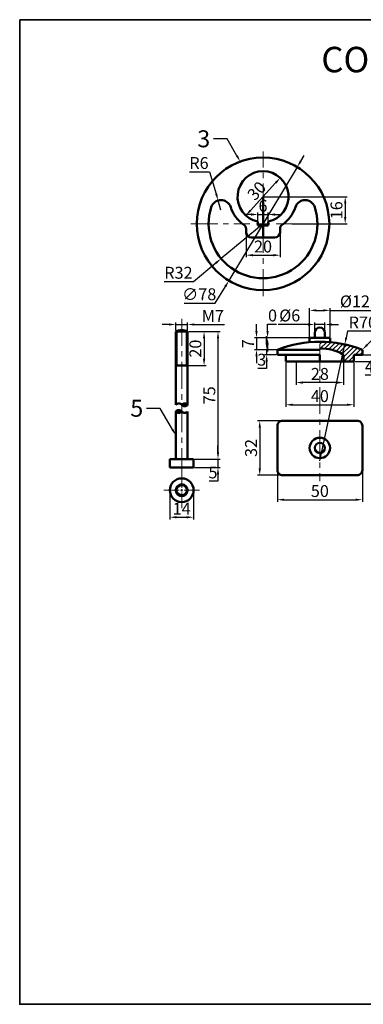
# Model space of a CAD drawing. Units: millimetres. Extents: x 214 to 813, y -258 to 321.
# Tile 1 of 4: x 214 to 416, y -258 to 321. Entities that reach past the tile are written whole.
import ezdxf
from ezdxf import colors
from ezdxf.entities.mleader import LeaderData, LeaderLine
from ezdxf.math import Vec2, Vec3

# ---------------------------------------------------------------- set-up
doc = ezdxf.new("R2010")
doc.units = ezdxf.units.MM
doc.header["$LTSCALE"] = 0.5
doc.linetypes.add('CENTER', pattern=[50.8, 31.75, -6.35, 6.35, -6.35])
for name, color, linetype, lineweight in [('M-CNTR', 1, 'CENTER', 18), ('M-DIMS', 2, 'Continuous', 25), ('M-HATC', 8, 'Continuous', 18), ('M-OUTL', 7, 'Continuous', 50), ('M-TTLB', 7, 'Continuous', 35)]:
    doc.layers.add(name, color=color, linetype=linetype, lineweight=lineweight)
doc.styles.get("Standard").update_dxf_attribs({"font": 'arial.ttf'})
doc.dimstyles.new('ISO-25', dxfattribs={"dimtxt": 7, "dimasz": 4, "dimexe": 1.25, "dimexo": 0.625, "dimtad": 1, "dimtoh": 1, "dimtxsty": 'Standard', "dimcen": 2.5, "dimadec": 0, "dimazin": 0, "dimtfac": 1, "dimtmove": 0, "dimatfit": 3, "dimfxl": 1, "dimarcsym": 0})
pattern_1 = [(45, (-3.20253, -20.17053), (-0.2245064, 0.2245064), [])]

# ---------------------------------------------------------------- blocks, each defined once
blk = doc.blocks.new('*U1')
at = {"layer": 'M-CNTR', "color": 0, "transparency": 16777216}
for p, q in [((0, 7.8), (0, 42.5)), ((-42.5, 0), (-7.8, 0)), ((7.8, 0), (42.5, 0)), ((0, -42.5), (0, -7.8))]:
    blk.add_line(p, q, dxfattribs=at)
at = {"layer": 'M-CNTR', "color": 0, "linetype": 'Continuous', "transparency": 16777216}
for p, q in [((-3.9, 0), (3.9, 0)), ((0, -3.9), (0, 3.9))]:
    blk.add_line(p, q, dxfattribs=at)
blk = doc.blocks.new('*D26')
at = {"layer": 'Defpoints', "color": 0, "ltscale": 0.5, "transparency": 16777216}
for p in [(367.44, 228.4), (347.21, 206.25), (347.21, 206.25)]:
    blk.add_point(p, dxfattribs=at)
at = {"layer": 'M-DIMS', "color": 0, "lineweight": -2, "ltscale": 0.5, "transparency": 16777216}
for p, q in [((366.98, 228.82), (366.52, 229.24)), ((364.75, 225.45), (349.91, 209.2)), ((346.75, 206.67), (346.29, 207.09))]:
    blk.add_line(p, q, dxfattribs=at)
at = {"layer": 'M-DIMS', "color": 0, "ltscale": 0.5, "transparency": 16777216}
for points in [[(364.25, 225.89), (365.24, 225), (367.44, 228.4)], [(349.42, 209.65), (350.4, 208.75), (347.21, 206.25)]]:
    blk.add_solid(points, dxfattribs=at)
at = {"layer": 'M-DIMS', "color": 0, "ltscale": 0.5, "transparency": 16777216, "insert": (354.23, 220.16), "char_height": 7, "attachment_point": 5, "rotation": 47.59957}
blk.add_mtext('30', dxfattribs=at)
blk = doc.blocks.new('*D27')
at = {"layer": 'Defpoints', "color": 0, "ltscale": 0.5, "transparency": 16777216}
for p in [(360.33, 206.82), (354.33, 202.63), (360.33, 202.63)]:
    blk.add_point(p, dxfattribs=at)
at = {"layer": 'M-DIMS', "color": 0, "lineweight": -2, "ltscale": 0.5, "transparency": 16777216}
for p, q in [((350.33, 206.82), (346.33, 206.82)), ((354.33, 203.25), (354.33, 208.07)), ((354.33, 206.82), (360.33, 206.82)), ((360.33, 203.25), (360.33, 208.07)), ((364.33, 206.82), (368.33, 206.82))]:
    blk.add_line(p, q, dxfattribs=at)
at = {"layer": 'M-DIMS', "color": 0, "ltscale": 0.5, "transparency": 16777216}
for points in [[(350.33, 207.49), (350.33, 206.16), (354.33, 206.82)], [(364.33, 207.49), (364.33, 206.16), (360.33, 206.82)]]:
    blk.add_solid(points, dxfattribs=at)
at = {"layer": 'M-DIMS', "color": 0, "ltscale": 0.5, "transparency": 16777216, "insert": (357.33, 211.02), "char_height": 7, "attachment_point": 5}
blk.add_mtext('6', dxfattribs=at)
blk = doc.blocks.new('*D28')
at = {"layer": 'Defpoints', "color": 0, "ltscale": 0.5, "transparency": 16777216}
for p in [(357.33, 201.32), (332.71, 180.88)]:
    blk.add_point(p, dxfattribs=at)
at = {"layer": 'M-DIMS', "color": 0, "lineweight": -2, "ltscale": 0.5, "transparency": 16777216}
for p, q in [((357.33, 201.32), (332.71, 180.88)), ((316.5, 167.42), (329.63, 178.32)), ((299.22, 167.42), (316.5, 167.42))]:
    blk.add_line(p, q, dxfattribs=at)
at = {"layer": 'M-DIMS', "color": 0, "ltscale": 0.5, "transparency": 16777216}
blk.add_solid([(329.21, 178.84), (330.06, 177.81), (332.71, 180.88)], dxfattribs=at)
at = {"layer": 'M-DIMS', "color": 0, "ltscale": 0.5, "transparency": 16777216, "insert": (307.55, 171.62), "char_height": 7, "attachment_point": 5}
blk.add_mtext('R32', dxfattribs=at)
blk = doc.blocks.new('*D29')
at = {"layer": 'Defpoints', "color": 0, "ltscale": 0.5, "transparency": 16777216}
for p in [(377.42, 234.75), (337.24, 167.89)]:
    blk.add_point(p, dxfattribs=at)
at = {"layer": 'M-DIMS', "color": 0, "lineweight": -2, "ltscale": 0.5, "transparency": 16777216}
for p, q in [((379.48, 238.18), (381.54, 241.61)), ((377.42, 234.75), (337.24, 167.89)), ((329.24, 154.57), (335.18, 164.46)), ((310.95, 154.57), (329.24, 154.57))]:
    blk.add_line(p, q, dxfattribs=at)
at = {"layer": 'M-DIMS', "color": 0, "ltscale": 0.5, "transparency": 16777216}
for points in [[(378.91, 238.52), (380.05, 237.84), (377.42, 234.75)], [(334.61, 164.81), (335.75, 164.12), (337.24, 167.89)]]:
    blk.add_solid(points, dxfattribs=at)
at = {"layer": 'M-DIMS', "color": 0, "ltscale": 0.5, "transparency": 16777216, "insert": (319.78, 158.97), "char_height": 7, "attachment_point": 5}
blk.add_mtext('∅78', dxfattribs=at)
blk = doc.blocks.new('*D30')
at = {"layer": 'Defpoints', "color": 0, "ltscale": 0.5, "transparency": 16777216}
for p in [(347.33, 196.32), (367.33, 196.32), (367.33, 182.87)]:
    blk.add_point(p, dxfattribs=at)
at = {"layer": 'M-DIMS', "color": 0, "lineweight": -2, "ltscale": 0.5, "transparency": 16777216}
for p, q in [((347.33, 195.7), (347.33, 181.62)), ((367.33, 195.7), (367.33, 181.62)), ((351.33, 182.87), (363.33, 182.87))]:
    blk.add_line(p, q, dxfattribs=at)
at = {"layer": 'M-DIMS', "color": 0, "ltscale": 0.5, "transparency": 16777216}
for points in [[(351.33, 183.54), (351.33, 182.21), (347.33, 182.87)], [(363.33, 183.54), (363.33, 182.21), (367.33, 182.87)]]:
    blk.add_solid(points, dxfattribs=at)
at = {"layer": 'M-DIMS', "color": 0, "ltscale": 0.5, "transparency": 16777216, "insert": (357.33, 187.07), "char_height": 7, "attachment_point": 5}
blk.add_mtext('20', dxfattribs=at)
blk = doc.blocks.new('*D31')
at = {"layer": 'Defpoints', "color": 0, "ltscale": 0.5, "transparency": 16777216}
for p in [(330.9, 215.08), (332.59, 209.32)]:
    blk.add_point(p, dxfattribs=at)
at = {"layer": 'M-DIMS', "color": 0, "lineweight": -2, "ltscale": 0.5, "transparency": 16777216}
for p, q in [((314, 232.03), (325.91, 232.03)), ((325.91, 232.03), (329.77, 218.92)), ((332.59, 209.32), (330.9, 215.08))]:
    blk.add_line(p, q, dxfattribs=at)
at = {"layer": 'M-DIMS', "color": 0, "ltscale": 0.5, "transparency": 16777216}
blk.add_solid([(330.41, 219.1), (329.13, 218.73), (330.9, 215.08)], dxfattribs=at)
at = {"layer": 'M-DIMS', "color": 0, "ltscale": 0.5, "transparency": 16777216, "insert": (319.64, 236.23), "char_height": 7, "attachment_point": 5}
blk.add_mtext('R6', dxfattribs=at)
blk = doc.blocks.new('*D32')
at = {"layer": 'Defpoints', "color": 0, "ltscale": 0.5, "transparency": 16777216}
for p in [(357.33, 217.32), (373.64, 201.32), (405.66, 201.32)]:
    blk.add_point(p, dxfattribs=at)
at = {"layer": 'M-DIMS', "color": 0, "lineweight": -2, "ltscale": 0.5, "transparency": 16777216}
for p, q in [((357.95, 217.32), (406.91, 217.32)), ((405.66, 213.32), (405.66, 205.32)), ((374.27, 201.32), (406.91, 201.32))]:
    blk.add_line(p, q, dxfattribs=at)
at = {"layer": 'M-DIMS', "color": 0, "ltscale": 0.5, "transparency": 16777216}
for points in [[(404.99, 213.32), (406.33, 213.32), (405.66, 217.32)], [(404.99, 205.32), (406.33, 205.32), (405.66, 201.32)]]:
    blk.add_solid(points, dxfattribs=at)
at = {"layer": 'M-DIMS', "color": 0, "ltscale": 0.5, "transparency": 16777216, "insert": (401.46, 209.32), "char_height": 7, "attachment_point": 5, "rotation": 90}
blk.add_mtext('16', dxfattribs=at)
blk = doc.blocks.new('*U37')
at = {"layer": 'M-CNTR', "color": 0, "transparency": 16777216}
blk.add_line((0, 6), (0, -6), dxfattribs=at)
blk = doc.blocks.new('*U38')
at = {"layer": 'M-CNTR', "color": 0, "transparency": 16777216}
blk.add_line((0, 48.82), (0, -33.73), dxfattribs=at)
blk = doc.blocks.new('*U40')
at = {"layer": 'M-CNTR', "color": 0, "transparency": 16777216}
for p, q in [((0, 1.4), (0, 10.5)), ((-10.5, 0), (-1.4, 0)), ((1.4, 0), (10.5, 0)), ((0, -10.5), (0, -1.4))]:
    blk.add_line(p, q, dxfattribs=at)
at = {"layer": 'M-CNTR', "color": 0, "linetype": 'Continuous', "transparency": 16777216}
for p, q in [((-0.7, 0), (0.7, 0)), ((0, -0.7), (0, 0.7))]:
    blk.add_line(p, q, dxfattribs=at)
blk = doc.blocks.new('*D41')
at = {"layer": 'Defpoints', "color": 0, "ltscale": 0.5, "transparency": 16777216}
for p in [(312.97, 137.88), (312.97, 117.88), (322.63, 117.88)]:
    blk.add_point(p, dxfattribs=at)
at = {"layer": 'M-DIMS', "color": 0, "lineweight": -2, "ltscale": 0.5, "transparency": 16777216}
for p, q in [((313.6, 137.88), (323.88, 137.88)), ((322.63, 133.88), (322.63, 121.88)), ((313.6, 117.88), (323.88, 117.88))]:
    blk.add_line(p, q, dxfattribs=at)
at = {"layer": 'M-DIMS', "color": 0, "ltscale": 0.5, "transparency": 16777216}
for points in [[(321.97, 133.88), (323.3, 133.88), (322.63, 137.88)], [(321.97, 121.88), (323.3, 121.88), (322.63, 117.88)]]:
    blk.add_solid(points, dxfattribs=at)
at = {"layer": 'M-DIMS', "color": 0, "ltscale": 0.5, "transparency": 16777216, "insert": (318.44, 127.88), "char_height": 7, "attachment_point": 5, "rotation": 90}
blk.add_mtext('20', dxfattribs=at)
blk = doc.blocks.new('*D42')
at = {"layer": 'Defpoints', "color": 0, "ltscale": 0.5, "transparency": 16777216}
for p in [(320.65, 137.88), (316.47, 62.88), (330.82, 62.88)]:
    blk.add_point(p, dxfattribs=at)
at = {"layer": 'M-DIMS', "color": 0, "lineweight": -2, "ltscale": 0.5, "transparency": 16777216}
for p, q in [((321.27, 137.88), (332.07, 137.88)), ((330.82, 133.88), (330.82, 66.88)), ((317.1, 62.88), (332.07, 62.88))]:
    blk.add_line(p, q, dxfattribs=at)
at = {"layer": 'M-DIMS', "color": 0, "ltscale": 0.5, "transparency": 16777216}
for points in [[(330.16, 133.88), (331.49, 133.88), (330.82, 137.88)], [(330.16, 66.88), (331.49, 66.88), (330.82, 62.88)]]:
    blk.add_solid(points, dxfattribs=at)
at = {"layer": 'M-DIMS', "color": 0, "ltscale": 0.5, "transparency": 16777216, "insert": (326.64, 100.38), "char_height": 7, "attachment_point": 5, "rotation": 90}
blk.add_mtext('75', dxfattribs=at)
blk = doc.blocks.new('*D43')
at = {"layer": 'Defpoints', "color": 0, "ltscale": 0.5, "transparency": 16777216}
for p in [(316.47, 62.88), (316.47, 57.88), (330.82, 57.88)]:
    blk.add_point(p, dxfattribs=at)
at = {"layer": 'M-DIMS', "color": 0, "lineweight": -2, "ltscale": 0.5, "transparency": 16777216}
for p, q in [((330.82, 66.88), (330.82, 70.88)), ((317.1, 62.88), (332.07, 62.88)), ((330.82, 62.88), (330.82, 57.88)), ((317.1, 57.88), (332.07, 57.88)), ((330.82, 53.88), (330.82, 49.88)), ((330.82, 49.88), (325.56, 49.88))]:
    blk.add_line(p, q, dxfattribs=at)
at = {"layer": 'M-DIMS', "color": 0, "ltscale": 0.5, "transparency": 16777216}
for points in [[(330.16, 66.88), (331.49, 66.88), (330.82, 62.88)], [(330.16, 53.88), (331.49, 53.88), (330.82, 57.88)]]:
    blk.add_solid(points, dxfattribs=at)
at = {"layer": 'M-DIMS', "color": 0, "ltscale": 0.5, "transparency": 16777216, "insert": (327.88, 54.07), "char_height": 7, "attachment_point": 5}
blk.add_mtext('5', dxfattribs=at)
blk = doc.blocks.new('*D44')
at = {"layer": 'Defpoints', "color": 0, "ltscale": 0.5, "transparency": 16777216}
for p in [(302.47, 44.51), (316.47, 44.51), (316.47, 28.61)]:
    blk.add_point(p, dxfattribs=at)
at = {"layer": 'M-DIMS', "color": 0, "lineweight": -2, "ltscale": 0.5, "transparency": 16777216}
for p, q in [((302.47, 43.89), (302.47, 27.36)), ((316.47, 43.89), (316.47, 27.36)), ((306.47, 28.61), (312.47, 28.61))]:
    blk.add_line(p, q, dxfattribs=at)
at = {"layer": 'M-DIMS', "color": 0, "ltscale": 0.5, "transparency": 16777216}
for points in [[(306.47, 29.28), (306.47, 27.94), (302.47, 28.61)], [(312.47, 29.28), (312.47, 27.94), (316.47, 28.61)]]:
    blk.add_solid(points, dxfattribs=at)
at = {"layer": 'M-DIMS', "color": 0, "ltscale": 0.5, "transparency": 16777216, "insert": (309.47, 32.75), "char_height": 7, "attachment_point": 5}
blk.add_mtext('14', dxfattribs=at)
blk = doc.blocks.new('*D45')
at = {"layer": 'Defpoints', "color": 0, "ltscale": 0.5, "transparency": 16777216}
for p in [(312.97, 142.08), (305.97, 137.88), (312.97, 137.88)]:
    blk.add_point(p, dxfattribs=at)
at = {"layer": 'M-DIMS', "color": 0, "lineweight": -2, "ltscale": 0.5, "transparency": 16777216}
for p, q in [((301.97, 142.08), (297.97, 142.08)), ((305.97, 138.51), (305.97, 143.33)), ((305.97, 142.08), (312.97, 142.08)), ((312.97, 138.51), (312.97, 143.33)), ((316.97, 142.08), (334.64, 142.08))]:
    blk.add_line(p, q, dxfattribs=at)
at = {"layer": 'M-DIMS', "color": 0, "ltscale": 0.5, "transparency": 16777216}
for points in [[(301.97, 142.74), (301.97, 141.41), (305.97, 142.08)], [(316.97, 142.74), (316.97, 141.41), (312.97, 142.08)]]:
    blk.add_solid(points, dxfattribs=at)
at = {"layer": 'M-DIMS', "color": 0, "ltscale": 0.5, "transparency": 16777216, "insert": (327.8, 146.2), "char_height": 7, "attachment_point": 5}
blk.add_mtext('M7', dxfattribs=at)
blk = doc.blocks.new('*U46')
at = {"layer": 'M-CNTR', "color": 0, "transparency": 16777216}
blk.add_line((0, 61.28), (0, -19.5), dxfattribs=at)
blk = doc.blocks.new('*D47')
at = {"layer": 'Defpoints', "color": 0, "ltscale": 0.5, "transparency": 16777216}
for p in [(396.75, 150.39), (384.75, 134.26), (396.75, 134.26)]:
    blk.add_point(p, dxfattribs=at)
at = {"layer": 'M-DIMS', "color": 0, "lineweight": -2, "ltscale": 0.5, "transparency": 16777216}
for p, q in [((384.75, 134.88), (384.75, 151.64)), ((396.75, 134.88), (396.75, 151.64)), ((388.75, 150.39), (392.75, 150.39)), ((396.75, 150.39), (420.79, 150.39))]:
    blk.add_line(p, q, dxfattribs=at)
at = {"layer": 'M-DIMS', "color": 0, "ltscale": 0.5, "transparency": 16777216}
for points in [[(388.75, 151.05), (388.75, 149.72), (384.75, 150.39)], [(392.75, 151.05), (392.75, 149.72), (396.75, 150.39)]]:
    blk.add_solid(points, dxfattribs=at)
at = {"layer": 'M-DIMS', "color": 0, "ltscale": 0.5, "transparency": 16777216, "insert": (411.38, 154.78), "char_height": 7, "attachment_point": 5}
blk.add_mtext('%%C12', dxfattribs=at)
blk = doc.blocks.new('*D48')
at = {"layer": 'Defpoints', "color": 0, "ltscale": 0.5, "transparency": 16777216}
for p in [(387.75, 142.08), (387.75, 135.76), (393.75, 135.76)]:
    blk.add_point(p, dxfattribs=at)
at = {"layer": 'M-DIMS', "color": 0, "lineweight": -2, "ltscale": 0.5, "transparency": 16777216}
for p, q in [((383.75, 142.08), (366.3, 142.08)), ((387.75, 136.38), (387.75, 143.33)), ((393.75, 142.08), (387.75, 142.08)), ((393.75, 136.38), (393.75, 143.33)), ((397.75, 142.08), (401.75, 142.08))]:
    blk.add_line(p, q, dxfattribs=at)
at = {"layer": 'M-DIMS', "color": 0, "ltscale": 0.5, "transparency": 16777216}
for points in [[(383.75, 142.75), (383.75, 141.42), (387.75, 142.08)], [(397.75, 142.75), (397.75, 141.42), (393.75, 142.08)]]:
    blk.add_solid(points, dxfattribs=at)
at = {"layer": 'M-DIMS', "color": 0, "ltscale": 0.5, "transparency": 16777216, "insert": (373.02, 146.48), "char_height": 7, "attachment_point": 5}
blk.add_mtext('%%C6', dxfattribs=at)
blk = doc.blocks.new('*D49')
at = {"layer": 'Defpoints', "color": 0, "ltscale": 0.5, "transparency": 16777216}
for p in [(370.75, 120.26), (410.75, 120.26), (410.75, 94.84)]:
    blk.add_point(p, dxfattribs=at)
at = {"layer": 'M-DIMS', "color": 0, "lineweight": -2, "ltscale": 0.5, "transparency": 16777216}
for p, q in [((370.75, 119.63), (370.75, 93.59)), ((410.75, 119.63), (410.75, 93.59)), ((374.75, 94.84), (406.75, 94.84))]:
    blk.add_line(p, q, dxfattribs=at)
at = {"layer": 'M-DIMS', "color": 0, "ltscale": 0.5, "transparency": 16777216}
for points in [[(374.75, 95.51), (374.75, 94.18), (370.75, 94.84)], [(406.75, 95.51), (406.75, 94.18), (410.75, 94.84)]]:
    blk.add_solid(points, dxfattribs=at)
at = {"layer": 'M-DIMS', "color": 0, "ltscale": 0.5, "transparency": 16777216, "insert": (390.75, 99.04), "char_height": 7, "attachment_point": 5}
blk.add_mtext('40', dxfattribs=at)
blk = doc.blocks.new('*D50')
at = {"layer": 'Defpoints', "color": 0, "ltscale": 0.5, "transparency": 16777216}
for p in [(360, 134.26), (390.75, 134.26), (390.75, 134.26)]:
    blk.add_point(p, dxfattribs=at)
at = {"layer": 'M-DIMS', "color": 0, "lineweight": -2, "ltscale": 0.5, "transparency": 16777216}
for p, q in [((360, 138.26), (360, 142.26)), ((360, 142.26), (365.19, 142.26)), ((390.12, 134.26), (358.75, 134.26)), ((390.12, 134.26), (358.75, 134.26)), ((360, 130.26), (360, 126.26))]:
    blk.add_line(p, q, dxfattribs=at)
at = {"layer": 'M-DIMS', "color": 0, "ltscale": 0.5, "transparency": 16777216}
for points in [[(359.34, 138.26), (360.67, 138.26), (360, 134.26)], [(359.34, 130.26), (360.67, 130.26), (360, 134.26)]]:
    blk.add_solid(points, dxfattribs=at)
at = {"layer": 'M-DIMS', "color": 0, "ltscale": 0.5, "transparency": 16777216, "insert": (362.91, 146.46), "char_height": 7, "attachment_point": 5}
blk.add_mtext('0', dxfattribs=at)
blk = doc.blocks.new('*D51')
at = {"layer": 'Defpoints', "color": 0, "ltscale": 0.5, "transparency": 16777216}
for p in [(384.75, 134.26), (353.47, 127.26), (384.75, 127.26)]:
    blk.add_point(p, dxfattribs=at)
at = {"layer": 'M-DIMS', "color": 0, "lineweight": -2, "ltscale": 0.5, "transparency": 16777216}
for p, q in [((353.47, 138.26), (353.47, 142.26)), ((384.12, 134.26), (352.22, 134.26)), ((353.47, 134.26), (353.47, 127.26)), ((384.12, 127.26), (352.22, 127.26)), ((353.47, 123.26), (353.47, 119.26))]:
    blk.add_line(p, q, dxfattribs=at)
at = {"layer": 'M-DIMS', "color": 0, "ltscale": 0.5, "transparency": 16777216}
for points in [[(352.81, 138.26), (354.14, 138.26), (353.47, 134.26)], [(352.81, 123.26), (354.14, 123.26), (353.47, 127.26)]]:
    blk.add_solid(points, dxfattribs=at)
at = {"layer": 'M-DIMS', "color": 0, "ltscale": 0.5, "transparency": 16777216, "insert": (349.35, 130.76), "char_height": 7, "attachment_point": 5, "rotation": 90}
blk.add_mtext('7', dxfattribs=at)
blk = doc.blocks.new('*D52')
at = {"layer": 'Defpoints', "color": 0, "ltscale": 0.5, "transparency": 16777216}
for p in [(359.46, 124.26), (365.75, 127.26), (365.75, 124.26)]:
    blk.add_point(p, dxfattribs=at)
at = {"layer": 'M-DIMS', "color": 0, "lineweight": -2, "ltscale": 0.5, "transparency": 16777216}
for p, q in [((359.46, 131.26), (359.46, 135.26)), ((365.12, 127.26), (358.21, 127.26)), ((365.12, 124.26), (358.21, 124.26)), ((359.46, 127.26), (359.46, 124.26)), ((359.46, 116.26), (354.26, 116.26)), ((359.46, 120.26), (359.46, 116.26))]:
    blk.add_line(p, q, dxfattribs=at)
at = {"layer": 'M-DIMS', "color": 0, "ltscale": 0.5, "transparency": 16777216}
for points in [[(358.8, 131.26), (360.13, 131.26), (359.46, 127.26)], [(358.8, 120.26), (360.13, 120.26), (359.46, 124.26)]]:
    blk.add_solid(points, dxfattribs=at)
at = {"layer": 'M-DIMS', "color": 0, "ltscale": 0.5, "transparency": 16777216, "insert": (356.55, 120.46), "char_height": 7, "attachment_point": 5}
blk.add_mtext('3', dxfattribs=at)
blk = doc.blocks.new('*D53')
at = {"layer": 'Defpoints', "color": 0, "ltscale": 0.5, "transparency": 16777216}
for p in [(410.75, 124.26), (410.75, 120.26), (422.94, 120.26)]:
    blk.add_point(p, dxfattribs=at)
at = {"layer": 'M-DIMS', "color": 0, "lineweight": -2, "ltscale": 0.5, "transparency": 16777216}
for p, q in [((422.94, 128.26), (422.94, 132.26)), ((411.37, 124.26), (424.19, 124.26)), ((422.94, 124.26), (422.94, 120.26)), ((411.37, 120.26), (424.19, 120.26)), ((422.94, 116.26), (422.94, 112.26)), ((422.94, 112.26), (417.48, 112.26))]:
    blk.add_line(p, q, dxfattribs=at)
at = {"layer": 'M-DIMS', "color": 0, "ltscale": 0.5, "transparency": 16777216}
for points in [[(422.28, 128.26), (423.61, 128.26), (422.94, 124.26)], [(422.28, 116.26), (423.61, 116.26), (422.94, 120.26)]]:
    blk.add_solid(points, dxfattribs=at)
at = {"layer": 'M-DIMS', "color": 0, "ltscale": 0.5, "transparency": 16777216, "insert": (419.9, 116.38), "char_height": 7, "attachment_point": 5}
blk.add_mtext('4', dxfattribs=at)
blk = doc.blocks.new('*D54')
at = {"layer": 'Defpoints', "color": 0, "ltscale": 0.5, "transparency": 16777216}
for p in [(376.75, 120.26), (404.75, 120.26), (376.75, 107.89)]:
    blk.add_point(p, dxfattribs=at)
at = {"layer": 'M-DIMS', "color": 0, "lineweight": -2, "ltscale": 0.5, "transparency": 16777216}
for p, q in [((376.75, 119.63), (376.75, 106.64)), ((404.75, 119.63), (404.75, 106.64)), ((400.75, 107.89), (380.75, 107.89))]:
    blk.add_line(p, q, dxfattribs=at)
at = {"layer": 'M-DIMS', "color": 0, "ltscale": 0.5, "transparency": 16777216}
for points in [[(380.75, 108.56), (380.75, 107.23), (376.75, 107.89)], [(400.75, 108.56), (400.75, 107.23), (404.75, 107.89)]]:
    blk.add_solid(points, dxfattribs=at)
at = {"layer": 'M-DIMS', "color": 0, "ltscale": 0.5, "transparency": 16777216, "insert": (390.75, 112.09), "char_height": 7, "attachment_point": 5}
blk.add_mtext('28', dxfattribs=at)
blk = doc.blocks.new('*D55')
at = {"layer": 'Defpoints', "color": 0, "ltscale": 0.5, "transparency": 16777216}
for p in [(405.38, 130.33), (390.75, 61.88)]:
    blk.add_point(p, dxfattribs=at)
at = {"layer": 'M-DIMS', "color": 0, "lineweight": -2, "ltscale": 0.5, "transparency": 16777216}
for p, q in [((407.06, 138.15), (406.22, 134.24)), ((424.38, 138.15), (407.06, 138.15)), ((390.75, 61.88), (405.38, 130.33))]:
    blk.add_line(p, q, dxfattribs=at)
at = {"layer": 'M-DIMS', "color": 0, "ltscale": 0.5, "transparency": 16777216}
blk.add_solid([(405.57, 134.38), (406.87, 134.1), (405.38, 130.33)], dxfattribs=at)
at = {"layer": 'M-DIMS', "color": 0, "ltscale": 0.5, "transparency": 16777216, "insert": (416.03, 142.35), "char_height": 7, "attachment_point": 5}
blk.add_mtext('R70', dxfattribs=at)
blk = doc.blocks.new('*D56')
at = {"layer": 'Defpoints', "color": 0, "ltscale": 0.5, "transparency": 16777216}
for p in [(365.75, 60.89), (415.75, 60.89), (415.75, 38.94)]:
    blk.add_point(p, dxfattribs=at)
at = {"layer": 'M-DIMS', "color": 0, "lineweight": -2, "ltscale": 0.5, "transparency": 16777216}
for p, q in [((365.75, 60.26), (365.75, 37.69)), ((415.75, 60.26), (415.75, 37.69)), ((369.75, 38.94), (411.75, 38.94))]:
    blk.add_line(p, q, dxfattribs=at)
at = {"layer": 'M-DIMS', "color": 0, "ltscale": 0.5, "transparency": 16777216}
for points in [[(369.75, 39.61), (369.75, 38.27), (365.75, 38.94)], [(411.75, 39.61), (411.75, 38.27), (415.75, 38.94)]]:
    blk.add_solid(points, dxfattribs=at)
at = {"layer": 'M-DIMS', "color": 0, "ltscale": 0.5, "transparency": 16777216, "insert": (390.75, 43.14), "char_height": 7, "attachment_point": 5}
blk.add_mtext('50', dxfattribs=at)
blk = doc.blocks.new('*D57')
at = {"layer": 'Defpoints', "color": 0, "ltscale": 0.5, "transparency": 16777216}
for p in [(374.18, 85.4), (355.39, 53.4), (374.18, 53.4)]:
    blk.add_point(p, dxfattribs=at)
at = {"layer": 'M-DIMS', "color": 0, "lineweight": -2, "ltscale": 0.5, "transparency": 16777216}
for p, q in [((373.55, 85.4), (354.14, 85.4)), ((355.39, 81.4), (355.39, 57.4)), ((373.55, 53.4), (354.14, 53.4))]:
    blk.add_line(p, q, dxfattribs=at)
at = {"layer": 'M-DIMS', "color": 0, "ltscale": 0.5, "transparency": 16777216}
for points in [[(354.73, 81.4), (356.06, 81.4), (355.39, 85.4)], [(354.73, 57.4), (356.06, 57.4), (355.39, 53.4)]]:
    blk.add_solid(points, dxfattribs=at)
at = {"layer": 'M-DIMS', "color": 0, "ltscale": 0.5, "transparency": 16777216, "insert": (351.19, 69.4), "char_height": 7, "attachment_point": 5, "rotation": 90}
blk.add_mtext('32', dxfattribs=at)
blk = doc.blocks.new('ECCENTRIC-SHEAVE-WEB')
at = {"ltscale": 0.5}
for p, q in [((32, 48), (32, 24)), ((22, 27), (22, 29.03)), ((42, 27), (42, 29.03)), ((32, 24), (25, 24)), ((32, 24), (39, 24))]:
    blk.add_line(p, q, dxfattribs=at)
for centre, radius, start, end in [((32, 32), 32, 162.07979, 17.92021), ((7.26, 40), 6, 17.92021, 162.07979), ((32, 48), 20, 197.92021, 235.58261), ((32, 48), 20, 304.41739, 342.07979), ((56.74, 40), 6, 17.92021, 162.07979), ((19, 29.03), 3, 0, 55.58261), ((45, 29.03), 3, 124.41739, 180), ((25, 27), 3, 180, 270), ((39, 27), 3, 270, 0)]:
    blk.add_arc(centre, radius, start, end, dxfattribs=at)
blk = doc.blocks.new('BOLT-HEAD')
at = {"ltscale": 0.5}
for p, q in [((14, 5), (0, 5)), ((0, 5), (0, 0)), ((14, 0), (14, 5)), ((0, 0), (14, 0))]:
    blk.add_line(p, q, dxfattribs=at)

msp = doc.modelspace()

# ---------------------------------------------------------------- hatches: boundary and pattern name
at = {"layer": 'M-HATC', "ltscale": 0.5}
h = msp.add_hatch(dxfattribs=at)
h.set_pattern_fill('ANSI31', color=256, scale=0.6)
h.set_pattern_definition([(45, (35.3025, -6.7986), (-1.347038, 1.347038), [])])
h.paths.add_polyline_path([(390.748, 131.876), (390.748, 127.915, -0.1549082), (404.748, 124.26), (404.748, 120.26), (410.748, 120.26), (410.748, 124.26), (415.748, 124.26), (415.748, 127.26, 0.0915564)])
h = msp.add_hatch(dxfattribs=at)
h.set_pattern_fill('ANSI31', color=256, scale=0.1)
h.set_pattern_definition(pattern_1)
h.paths.add_polyline_path([(312.971, 94.81, 0.4793727), (309.471, 94.81, 0.4793727)])
h = msp.add_hatch(dxfattribs=at)
h.set_pattern_fill('ANSI31', color=256, scale=0.1)
h.set_pattern_definition(pattern_1)
h.paths.add_polyline_path([(305.971, 90.887, 0.4793727), (309.471, 90.887, 0.4793727)])

# ---------------------------------------------------------------- linework, layer by layer
at = {"layer": 'M-OUTL', "ltscale": 0.5}
for p, q in [((354.329, 200.322), (354.329, 202.625)), ((360.329, 200.322), (354.329, 200.322)), ((360.329, 202.625), (360.329, 200.322)), ((312.971, 137.884), (305.971, 137.884)), ((305.971, 137.884), (305.971, 94.81)), ((306.471, 137.884), (306.471, 117.884)), ((312.471, 117.884), (312.471, 137.884)), ((312.971, 94.81), (312.971, 137.884)), ((384.748, 134.26), (396.748, 134.26)), ((384.748, 134.26), (384.748, 131.619)), ((387.748, 137.26), (387.748, 134.26)), ((393.748, 134.26), (393.748, 137.26)), ((396.748, 134.26), (396.748, 131.619)), ((365.748, 124.26), (365.748, 127.26)), ((365.748, 127.26), (390.748, 127.26)), ((370.748, 124.26), (365.748, 124.26)), ((370.748, 120.26), (370.748, 124.26)), ((370.748, 124.26), (390.748, 124.26)), ((390.748, 124.26), (390.748, 120.26)), ((404.748, 124.26), (404.748, 120.26)), ((410.748, 124.26), (410.748, 120.26)), ((415.748, 124.26), (410.748, 124.26)), ((415.748, 127.26), (415.748, 124.26)), ((312.971, 117.884), (305.971, 117.884)), ((390.748, 120.26), (370.748, 120.26)), ((410.748, 120.26), (390.748, 120.26)), ((305.971, 90.887), (305.971, 62.884)), ((312.971, 62.884), (312.971, 90.887))]:
    msp.add_line(p, q, dxfattribs=at)
msp.add_lwpolyline([(415.748, 56.396), (415.748, 82.396, 0.4142136), (412.748, 85.396), (368.748, 85.396, 0.4142136), (365.748, 82.396), (365.748, 56.396, 0.4142136), (368.748, 53.396), (412.748, 53.396, 0.4142136)], format="xyb", close=True, dxfattribs=at)
for centre, radius in [((357.329, 201.322), 39), ((390.748, 69.396), 6), ((390.748, 69.396), 3), ((309.471, 44.512), 7), ((309.471, 44.512), 3.5), ((309.471, 44.512), 3)]:
    msp.add_circle(centre, radius, dxfattribs=at)
for centre, radius, start, end in [((357.329, 217.322), 15, 281.536959, 258.463041), ((390.748, 137.26), 3, 0, 180), ((309.471, 132.145), 6.722, 58.621567, 121.378433), ((390.748, 61.876), 70, 69.075168, 110.924832), ((391.991, 104.035), 23.912, 57.756989, 92.979383), ((307.721, 93.404), 2.245, 38.776426, 141.223574), ((311.221, 93.404), 2.245, 38.776426, 141.223574), ((311.221, 96.216), 2.245, 218.776426, 321.223574), ((307.721, 89.481), 2.245, 38.776426, 141.223574), ((307.721, 92.293), 2.245, 218.776426, 321.223574), ((311.221, 92.293), 2.245, 218.776426, 321.223574)]:
    msp.add_arc(centre, radius, start, end, dxfattribs=at)
at = {"layer": 'M-TTLB', "ltscale": 0.5}
msp.add_lwpolyline([(214.186, 321.5), (812.717, 321.5), (812.717, -258.089), (214.186, -258.089)], close=True, dxfattribs=at)

# ---------------------------------------------------------------- block references
at = {"layer": 'M-CNTR'}
for name, p in [('*U1', (357.329, 201.322)), ('*U38', (309.471, 96.616)), ('*U46', (390.748, 69.396)), ('*U37', (309.471, 60.384)), ('*U40', (309.471, 44.512))]:
    msp.add_blockref(name, p, dxfattribs=at)
at = {"layer": 'M-OUTL'}
for name, p in [('ECCENTRIC-SHEAVE-WEB', (325.327, 169.322)), ('BOLT-HEAD', (302.471, 57.884))]:
    msp.add_blockref(name, p, dxfattribs=at)

# ---------------------------------------------------------------- texts
at = {"layer": 'M-TTLB', "ltscale": 0.5, "insert": (391.608, 305.53), "char_height": 15, "attachment_point": 1}
msp.add_mtext_dynamic_manual_height_columns('COLLAR WITH ECCENTRIC ', width=324.14999, gutter_width=12.5, heights=[0], dxfattribs=at)

# ---------------------------------------------------------------- dimensions: what is measured, and where the dimension line sits
at = {"layer": 'M-DIMS', "ltscale": 0.5}
dim = msp.add_diameter_dim_2p(p1=(377.416, 234.751), p2=(337.241, 167.893), dimstyle='ISO-25', override={"dimclrd": 0, "dimclre": 0, "dimclrt": 0}, dxfattribs=at)
dim.commit()
dim.dimension.update_dxf_attribs({"geometry": '*D29', "text_midpoint": (319.783, 158.968)})
for center, mpoint, picture, middle in [((332.59, 209.322), (330.896, 215.078), '*D31', (319.639, 232.033)), ((357.329, 201.322), (332.711, 180.878), '*D28', (307.547, 167.415))]:
    dim = msp.add_radius_dim(center=center, mpoint=mpoint, dimstyle='ISO-25', override={"dimclrd": 0, "dimclre": 0, "dimclrt": 0}, dxfattribs=at)
    dim.commit()
    dim.dimension.update_dxf_attribs({"geometry": picture, "text_midpoint": middle, "dimtype": 164})
dim = msp.add_aligned_dim(p1=(367.443, 228.399), p2=(347.214, 206.245), distance=0, dimstyle='ISO-25', override={"dimclrd": 0, "dimclre": 0, "dimclrt": 0}, dxfattribs=at)
dim.commit()
dim.dimension.update_dxf_attribs({"geometry": '*D26', "text_midpoint": (354.226, 220.155)})
for base, p1, p2, angle, picture, middle, dimtype in [((360.329, 206.824), (354.329, 202.625), (360.329, 202.625), 0, '*D27', (357.329, 206.824), 161), ((360.002956191, 134.259664682), (390.748103932, 134.259664682), (390.748103932, 134.259664682), 90, '*D50', (362.910357282, 142.259664682), 160), ((353.472, 127.26), (384.748, 134.26), (384.748, 127.26), 90, '*D51', (353.472, 130.76), 160)]:
    dim = msp.add_linear_dim(base=base, p1=p1, p2=p2, angle=angle, dimstyle='ISO-25', override={"dimclrd": 0, "dimclre": 0, "dimclrt": 0}, dxfattribs=at)
    dim.commit()
    dim.dimension.update_dxf_attribs({"geometry": picture, "text_midpoint": middle, "dimtype": dimtype})
for base, p1, p2, picture, middle in [((405.659, 201.322), (357.329, 217.322), (373.643, 201.322), '*D32', (401.46, 209.322)), ((322.634, 117.884), (312.971, 137.884), (312.971, 117.884), '*D41', (318.435, 127.884)), ((330.823, 62.884), (320.645, 137.884), (316.471, 62.884), '*D42', (326.638, 100.384)), ((359.465, 124.26), (365.748, 127.26), (365.748, 124.26), '*D52', (356.548, 120.461)), ((422.944, 120.26), (410.748, 124.26), (410.748, 120.26), '*D53', (419.898, 116.385)), ((355.395, 53.396), (374.176, 85.396), (374.176, 53.396), '*D57', (351.194, 69.396)), ((330.823, 57.884), (316.471, 62.884), (316.471, 57.884), '*D43', (327.877, 54.068))]:
    dim = msp.add_linear_dim(base=base, p1=p1, p2=p2, angle=90, dimstyle='ISO-25', override={"dimclrd": 0, "dimclre": 0, "dimclrt": 0}, dxfattribs=at)
    dim.commit()
    dim.dimension.update_dxf_attribs({"geometry": picture, "text_midpoint": middle})
for base, p1, p2, picture, middle in [((367.329, 182.874), (347.329, 196.322), (367.329, 196.322), '*D30', (357.329, 187.073)), ((415.748, 38.939), (365.748, 60.888), (415.748, 60.888), '*D56', (390.748, 43.138)), ((316.471, 28.611), (302.471, 44.512), (316.471, 44.512), '*D44', (309.471, 32.75))]:
    dim = msp.add_linear_dim(base=base, p1=p1, p2=p2, dimstyle='ISO-25', override={"dimclrd": 0, "dimclre": 0, "dimclrt": 0}, dxfattribs=at)
    dim.commit()
    dim.dimension.update_dxf_attribs({"geometry": picture, "text_midpoint": middle})
for base, p1, p2, picture, middle in [((396.748, 150.387), (384.748, 134.26), (396.748, 134.26), '*D47', (411.38, 150.387)), ((387.748, 142.082), (393.748, 135.76), (387.748, 135.76), '*D48', (373.023, 142.082))]:
    dim = msp.add_linear_dim(base=base, p1=p1, p2=p2, text='%%C<>', dimstyle='ISO-25', override={"dimclrd": 0, "dimclre": 0, "dimclrt": 0}, dxfattribs=at)
    dim.commit()
    dim.dimension.update_dxf_attribs({"geometry": picture, "text_midpoint": middle, "dimtype": 160})
dim = msp.add_linear_dim(base=(312.971, 142.076), p1=(305.971, 137.884), p2=(312.971, 137.884), text='M<>', dimstyle='ISO-25', override={"dimclrd": 0, "dimclre": 0, "dimclrt": 0}, dxfattribs=at)
dim.commit()
dim.dimension.update_dxf_attribs({"geometry": '*D45', "text_midpoint": (327.803, 146.201)})
dim = msp.add_radius_dim(center=(390.748, 61.876), mpoint=(405.383, 130.329), dimstyle='ISO-25', override={"dimclrd": 0, "dimclre": 0, "dimclrt": 0}, dxfattribs=at)
dim.commit()
dim.dimension.update_dxf_attribs({"geometry": '*D55', "text_midpoint": (416.032, 142.351)})
for base, p1, p2, picture, middle in [((410.748, 94.842), (370.748, 120.26), (410.748, 120.26), '*D49', (390.748, 94.842)), ((376.748, 107.893), (404.748, 120.26), (376.748, 120.26), '*D54', (390.748, 107.893))]:
    dim = msp.add_linear_dim(base=base, p1=p1, p2=p2, dimstyle='ISO-25', override={"dimclrd": 0, "dimclre": 0, "dimclrt": 0}, dxfattribs=at)
    dim.commit()
    dim.dimension.update_dxf_attribs({"geometry": picture, "text_midpoint": middle, "dimtype": 160})

# ---------------------------------------------------------------- leaders
ml = msp.add_multileader_mtext('Standard', dxfattribs=at)
ml.set_content('3', color=256)
ml.set_leader_properties()
ml.build(insert=Vec2(0, 0))
ctx = ml.context
ctx.base_point, ctx.char_height, ctx.plane_origin = Vec3(317.684, 251.316), 10, Vec3(343.947, 237.954)
ctx.text_align_type = 2
notes = []
notes.append((ctx, [(0, (1, 1, 0), (336.233, 251.316), (-1, 0), 8, [(0, [(343.947, 237.954)], 0, [])])]))
ctx.mtext.insert, ctx.mtext.alignment, ctx.mtext.flow_direction = Vec3(326.233, 256.404), 3, 5
ml = msp.add_multileader_mtext('Standard', dxfattribs=at)
ml.set_content('4', color=256)
ml.set_leader_properties()
ml.build(insert=Vec2(0, 0))
ctx = ml.context
ctx.base_point, ctx.char_height, ctx.plane_origin = Vec3(440.235, 143.705), 10, Vec3(415.748, 127.26)
notes.append((ctx, [(0, (1, 1, 0), (432.235, 143.705), (1, 0), 8, [(0, [(415.748, 127.26)], 0, [])])]))
ctx.mtext.insert, ctx.mtext.flow_direction = Vec3(442.235, 148.705), 5
ml = msp.add_multileader_mtext('Standard', dxfattribs=at)
ml.set_content('5', color=256)
ml.set_leader_properties()
ml.build(insert=Vec2(0, 0))
ctx = ml.context
ctx.base_point, ctx.char_height, ctx.plane_origin = Vec3(278.203, 92.711), 10, Vec3(305.971, 76.885)
ctx.text_align_type = 2
notes.append((ctx, [(0, (1, 1, 0), (296.833, 92.711), (-1, 0), 8, [(0, [(305.971, 76.885)], 0, [])])]))
ctx.mtext.insert, ctx.mtext.alignment, ctx.mtext.flow_direction = Vec3(286.833, 97.797), 3, 5
for ctx, leaders in notes:
    for number, flags, end, landing, length, lines in leaders:
        leader = LeaderData()
        leader.index, (leader.has_last_leader_line, leader.has_dogleg_vector, leader.attachment_direction) = number, flags
        leader.last_leader_point, leader.dogleg_vector, leader.dogleg_length = Vec3(end), Vec3(landing), length
        for number, points, colour, breaks in lines:
            line = LeaderLine()
            line.index, line.vertices, line.color, line.breaks = number, Vec3.list(points), colors.encode_raw_color(colour), breaks
            leader.lines.append(line)
        ctx.leaders.append(leader)

doc.saveas('drawing.dxf')
